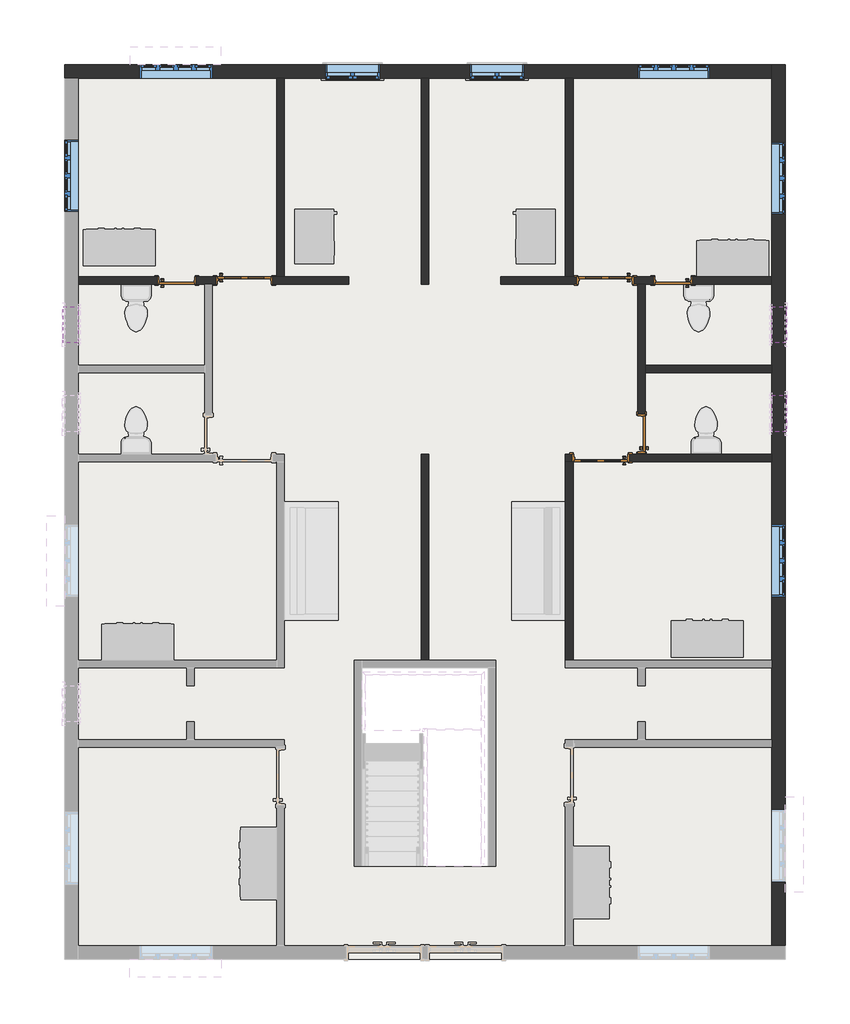
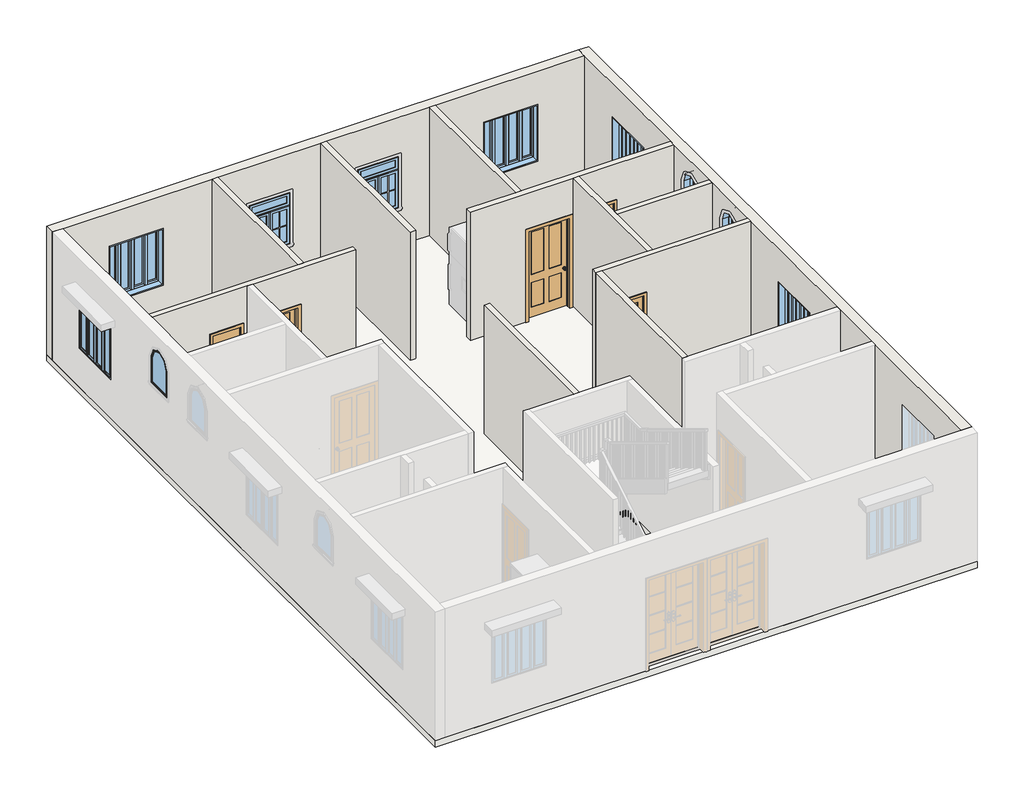
# One storey, part 2 of 4: 12 walls, 10 windows, 6 doors, 1 slab.
"""IFC4 building model written with IfcOpenShell, lengths in millimetres."""

from ifc_helpers import new_model, si_unit, frame, origin, origin_with_axes, place, context, project, spatial, polyline, circle_curve, outline, extrude, faceted_brep, transform, mapped, element, save
from ifc_brep_helpers import plane_surface, revolved_surface, advanced_brep
from components import door_a823658d, door_68a706ac, door_3f5f64ee, door_428b1ac9, window_casement_double_transom_0fae6a54, window_casement_multi_sash_horizontal_main_windows_4_x_7_0e27d311, window_2fd4accf

model = new_model("IFC4")

# Units and contexts
model_context = context("Model", 3, world=origin())
ifc_project = project(units=[si_unit("LENGTHUNIT", "METRE", prefix="MILLI")], contexts=[model_context])

# Site, building, storey
site = spatial("IfcSite", under=ifc_project)
building = spatial("IfcBuilding", under=site)
storey = spatial("IfcBuildingStorey", under=building, Elevation=0.0)

# Doors
placement = place(None, origin())
door_shape = door_a823658d(model_context)
element("IfcDoor", 1, ObjectType="Door-Interior-Single-4_Panel-Wood : 36\" x 84\"", at=placement, inside=storey, context=model_context, shape_type="MappedRepresentation", body=[
    mapped(door_shape, transform((-6490.9771954, 4939.0022103, 0.0), x_axis=(-1.0, 0.0, 0.0), y_axis=(0.0, -1.0, 0.0), z_axis=(0.0, 0.0, 1.0))),
])
door_2_shape = door_68a706ac(model_context)
element("IfcDoor", 2, ObjectType="Door-Interior-Single-4_Panel-Wood : 36\" x 84\"", at=placement, inside=storey, context=model_context, shape_type="MappedRepresentation", body=[
    mapped(door_2_shape, transform((-6567.1771954, 1935.9816069, 0.0), x_axis=(-1.0, 0.0, 0.0), y_axis=(0.0, -1.0, 0.0), z_axis=(0.0, 0.0, 1.0))),
])
element("IfcDoor", 3, ObjectType="Door-Interior-Single-4_Panel-Wood : 36\" x 84\"", at=placement, inside=storey, context=model_context, shape_type="MappedRepresentation", body=[
    mapped(door_2_shape, transform((-12586.9771954, 4939.0022103, 0.0), x_axis=(1.0, 0.0, 0.0), y_axis=(0.0, 1.0, 0.0), z_axis=(0.0, 0.0, 1.0))),
])
door_3_shape = door_3f5f64ee(model_context)
element("IfcDoor", 4, ObjectType="Door-Interior-Single-Flush_Panel-Wood : 24\" x 84\"", at=placement, inside=storey, context=model_context, shape_type="MappedRepresentation", body=[
    mapped(door_3_shape, transform((-5347.9771954, 4932.6522103, 0.0), x_axis=(-1.0, 0.0, 0.0), y_axis=(0.0, -1.0, 0.0), z_axis=(0.0, 0.0, 1.0))),
])
door_4_shape = door_428b1ac9(model_context)
element("IfcDoor", 5, ObjectType="Door-Interior-Single-Flush_Panel-Wood : 24\" x 84\"", at=placement, inside=storey, context=model_context, shape_type="MappedRepresentation", body=[
    mapped(door_4_shape, transform((-13729.9771954, 4932.6522103, 0.0), x_axis=(1.0, 0.0, 0.0), y_axis=(0.0, 1.0, 0.0), z_axis=(0.0, 0.0, 1.0))),
])
element("IfcDoor", 6, ObjectType="Door-Interior-Single-Flush_Panel-Wood : 24\" x 84\"", at=placement, inside=storey, context=model_context, shape_type="MappedRepresentation", body=[
    mapped(door_4_shape, transform((-5878.2021954, 2345.5566069, 0.0), x_axis=(0.0, 1.0, 0.0), y_axis=(-1.0, 0.0, 0.0), z_axis=(0.0, 0.0, 1.0))),
])

# Slab
element("IfcSlab", 7, ObjectType="MARBLE FLOORING 6\"", at=placement, inside=storey, context=model_context, shape_type="SweptSolid", body=[
    extrude(outline(polyline([(-3455.6771954, 8580.7272103), (-3455.6771954, -6532.2727897), (-15623.8646954, -6532.2727897), (-15623.8646954, 8580.7272103), (-3455.6771954, 8580.7272103)]), holes=[polyline([(-10605.7771954, -4957.4727897), (-8472.1771954, -4957.4727897), (-8472.1771954, -1604.6727897), (-10605.7771954, -1604.6727897), (-10605.7771954, -4957.4727897)])]), frame((0.0, 0.0, -152.4), z_axis=(0.0, 0.0, 1.0), x_axis=(1.0, 0.0, 0.0)), (0.0, 0.0, 1.0), 152.4),
])

# Walls
element("IfcWall", 8, ObjectType="INNER WALL 5\"", at=placement, inside=storey, context=model_context, shape_type="Brep", body=[
    faceted_brep([(-10821.6771954, 4872.3272103, 0.0), (-10821.6771954, 4872.3272103, 3048.0), (-13133.0771954, 4872.3272103, 3048.0), (-13260.0771954, 4872.3272103, 3048.0), (-15395.2646954, 4872.3272103, 3048.0), (-15395.2646954, 4872.3272103, 0.0), (-14060.1771954, 4872.3272103, 0.0), (-14060.1771954, 4872.3272103, 2159.0), (-13399.7771954, 4872.3272103, 2159.0), (-13399.7771954, 4872.3272103, 0.0), (-13260.0771954, 4872.3272103, 0.0), (-13133.0771954, 4872.3272103, 0.0), (-13069.5771954, 4872.3272103, 0.0), (-13069.5771954, 4872.3272103, 2159.0), (-12104.3771954, 4872.3272103, 2159.0), (-12104.3771954, 4872.3272103, 0.0), (-10821.6771954, 4999.3272103, 3048.0), (-10821.6771954, 4999.3272103, 0.0), (-11913.8771954, 4999.3272103, 0.0), (-12040.8771954, 4999.3272103, 0.0), (-12104.3771954, 4999.3272103, 0.0), (-12104.3771954, 4999.3272103, 2159.0), (-13069.5771954, 4999.3272103, 2159.0), (-13069.5771954, 4999.3272103, 0.0), (-13399.7771954, 4999.3272103, 0.0), (-13399.7771954, 4999.3272103, 2159.0), (-14060.1771954, 4999.3272103, 2159.0), (-14060.1771954, 4999.3272103, 0.0), (-15395.2646954, 4999.3272103, 0.0), (-15395.2646954, 4999.3272103, 3048.0), (-12040.8771954, 4999.3272103, 3048.0), (-11913.8771954, 4999.3272103, 3048.0)], [[[0, 1, 2, 3, 4, 5, 6, 7, 8, 9, 10, 11, 12, 13, 14, 15]], [[16, 17, 18, 19, 20, 21, 22, 23, 24, 25, 26, 27, 28, 29, 30, 31]], [[17, 0, 15, 20, 19, 18]], [[5, 28, 27, 6]], [[23, 12, 11, 10, 9, 24]], [[1, 0, 17, 16]], [[5, 4, 29, 28]], [[14, 21, 20, 15]], [[21, 14, 13, 22]], [[22, 13, 12, 23]], [[8, 25, 24, 9]], [[25, 8, 7, 26]], [[26, 7, 6, 27]], [[4, 3, 2, 1, 16, 31, 30, 29]]]),
])
element("IfcWall", 9, ObjectType="INNER WALL 5\"", at=placement, inside=storey, context=model_context, shape_type="Brep", body=[
    faceted_brep([(-8256.2771954, 4872.3272103, 3048.0), (-8256.2771954, 4872.3272103, 0.0), (-6973.5771954, 4872.3272103, 0.0), (-6973.5771954, 4872.3272103, 2159.0), (-6008.3771954, 4872.3272103, 2159.0), (-6008.3771954, 4872.3272103, 0.0), (-5944.8771954, 4872.3272103, 0.0), (-5817.8771954, 4872.3272103, 0.0), (-5678.1771954, 4872.3272103, 0.0), (-5678.1771954, 4872.3272103, 2159.0), (-5017.7771954, 4872.3272103, 2159.0), (-5017.7771954, 4872.3272103, 0.0), (-3684.2771954, 4872.3272103, 0.0), (-3684.2771954, 4872.3272103, 3048.0), (-5817.8771954, 4872.3272103, 3048.0), (-5944.8771954, 4872.3272103, 3048.0), (-8256.2771954, 4999.3272103, 0.0), (-8256.2771954, 4999.3272103, 3048.0), (-7164.0771954, 4999.3272103, 3048.0), (-7037.0771954, 4999.3272103, 3048.0), (-3684.2771954, 4999.3272103, 3048.0), (-3684.2771954, 4999.3272103, 0.0), (-5017.7771954, 4999.3272103, 0.0), (-5017.7771954, 4999.3272103, 2159.0), (-5678.1771954, 4999.3272103, 2159.0), (-5678.1771954, 4999.3272103, 0.0), (-6008.3771954, 4999.3272103, 0.0), (-6008.3771954, 4999.3272103, 2159.0), (-6973.5771954, 4999.3272103, 2159.0), (-6973.5771954, 4999.3272103, 0.0), (-7037.0771954, 4999.3272103, 0.0), (-7164.0771954, 4999.3272103, 0.0)], [[[0, 1, 2, 3, 4, 5, 6, 7, 8, 9, 10, 11, 12, 13, 14, 15]], [[16, 17, 18, 19, 20, 21, 22, 23, 24, 25, 26, 27, 28, 29, 30, 31]], [[1, 16, 31, 30, 29, 2]], [[21, 12, 11, 22]], [[5, 26, 25, 8, 7, 6]], [[1, 0, 17, 16]], [[13, 12, 21, 20]], [[28, 3, 2, 29]], [[3, 28, 27, 4]], [[4, 27, 26, 5]], [[24, 9, 8, 25]], [[9, 24, 23, 10]], [[10, 23, 22, 11]], [[0, 15, 14, 13, 20, 19, 18, 17]]]),
])
element("IfcWall", 10, ObjectType="INNER WALL 5\"", at=placement, inside=storey, context=model_context, shape_type="SweptSolid", body=[
    extrude(outline(polyline([(-12040.8771954, 4999.3272103), (-12040.8771954, 8352.1272103), (-11913.8771954, 8352.1272103), (-11913.8771954, 4999.3272103), (-12040.8771954, 4999.3272103)])), origin_with_axes(), (0.0, 0.0, 1.0), 3048.0),
])
element("IfcWall", 11, ObjectType="INNER WALL 5\"", at=placement, inside=storey, context=model_context, shape_type="SweptSolid", body=[
    extrude(outline(polyline([(-9602.4771954, 4872.3272103), (-9602.4771954, 8352.1272103), (-9475.4771954, 8352.1272103), (-9475.4771954, 4872.3272103), (-9602.4771954, 4872.3272103)])), origin_with_axes(), (0.0, 0.0, 1.0), 3048.0),
])
element("IfcWall", 12, ObjectType="INNER WALL 5\"", at=placement, inside=storey, context=model_context, shape_type="SweptSolid", body=[
    extrude(outline(polyline([(-7164.0771954, 4999.3272103), (-7164.0771954, 8352.1272103), (-7037.0771954, 8352.1272103), (-7037.0771954, 4999.3272103), (-7164.0771954, 4999.3272103)])), origin_with_axes(), (0.0, 0.0, 1.0), 3048.0),
])
element("IfcWall", 13, ObjectType="INNER WALL 5\"", at=placement, inside=storey, context=model_context, shape_type="SweptSolid", body=[
    extrude(outline(polyline([(-9602.4771954, -1477.6727897), (-9602.4771954, 2002.6566069), (-9475.4771954, 2002.6566069), (-9475.4771954, -1477.6727897), (-9602.4771954, -1477.6727897)])), origin_with_axes(), (0.0, 0.0, 1.0), 3048.0),
])
element("IfcWall", 14, ObjectType="INNER WALL 5\"", at=placement, inside=storey, context=model_context, shape_type="Brep", body=[
    faceted_brep([(-5944.8771954, 4872.3272103, 3048.0), (-5944.8771954, 4872.3272103, 0.0), (-5944.8771954, 2675.7566069, 0.0), (-5944.8771954, 2675.7566069, 2159.0), (-5944.8771954, 2015.3566069, 2159.0), (-5944.8771954, 2015.3566069, 0.0), (-5944.8771954, 2002.6566069, 0.0), (-5944.8771954, 2002.6566069, 3048.0), (-5817.8771954, 4872.3272103, 0.0), (-5817.8771954, 4872.3272103, 3048.0), (-5817.8771954, 3500.7272103, 3048.0), (-5817.8771954, 3373.7272103, 3048.0), (-5817.8771954, 2002.6566069, 3048.0), (-5817.8771954, 2002.6566069, 0.0), (-5817.8771954, 2015.3566069, 0.0), (-5817.8771954, 2015.3566069, 2159.0), (-5817.8771954, 2675.7566069, 2159.0), (-5817.8771954, 2675.7566069, 0.0), (-5817.8771954, 3373.7272103, 0.0), (-5817.8771954, 3500.7272103, 0.0)], [[[0, 1, 2, 3, 4, 5, 6, 7]], [[8, 9, 10, 11, 12, 13, 14, 15, 16, 17, 18, 19]], [[1, 8, 19, 18, 17, 2]], [[13, 6, 5, 14]], [[1, 0, 9, 8]], [[7, 6, 13, 12]], [[16, 3, 2, 17]], [[3, 16, 15, 4]], [[4, 15, 14, 5]], [[0, 7, 12, 11, 10, 9]]]),
])
element("IfcWall", 15, ObjectType="INNER WALL 5\"", at=placement, inside=storey, context=model_context, shape_type="SweptSolid", body=[
    extrude(outline(polyline([(-3684.2771954, 3373.7272103), (-5817.8771954, 3373.7272103), (-5817.8771954, 3500.7272103), (-3684.2771954, 3500.7272103), (-3684.2771954, 3373.7272103)])), origin_with_axes(), (0.0, 0.0, 1.0), 3048.0),
])
element("IfcWall", 16, ObjectType="INNER WALL 5\"", at=placement, inside=storey, context=model_context, shape_type="Brep", body=[
    faceted_brep([(-3684.2771954, 2002.6566069, 3048.0), (-3684.2771954, 2002.6566069, 0.0), (-5817.8771954, 2002.6566069, 0.0), (-5944.8771954, 2002.6566069, 0.0), (-6084.5771954, 2002.6566069, 0.0), (-6084.5771954, 2002.6566069, 2159.0), (-7049.7771954, 2002.6566069, 2159.0), (-7049.7771954, 2002.6566069, 0.0), (-7164.0771954, 2002.6566069, 0.0), (-7164.0771954, 2002.6566069, 3048.0), (-5944.8771954, 2002.6566069, 3048.0), (-5817.8771954, 2002.6566069, 3048.0), (-3684.2771954, 1875.6566069, 0.0), (-3684.2771954, 1875.6566069, 3048.0), (-7037.0771954, 1875.6566069, 3048.0), (-7164.0771954, 1875.6566069, 3048.0), (-7164.0771954, 1875.6566069, 0.0), (-7049.7771954, 1875.6566069, 0.0), (-7049.7771954, 1875.6566069, 2159.0), (-6084.5771954, 1875.6566069, 2159.0), (-6084.5771954, 1875.6566069, 0.0)], [[[0, 1, 2, 3, 4, 5, 6, 7, 8, 9, 10, 11]], [[12, 13, 14, 15, 16, 17, 18, 19, 20]], [[1, 12, 20, 4, 3, 2]], [[16, 8, 7, 17]], [[1, 0, 13, 12]], [[9, 8, 16, 15]], [[6, 18, 17, 7]], [[18, 6, 5, 19]], [[19, 5, 4, 20]], [[0, 11, 10, 9, 15, 14, 13]]]),
])
element("IfcWall", 17, ObjectType="INNER WALL 5\"", at=placement, inside=storey, context=model_context, shape_type="SweptSolid", body=[
    extrude(outline(polyline([(-7037.0771954, 1875.6566069), (-7037.0771954, -1477.6727897), (-7164.0771954, -1477.6727897), (-7164.0771954, 1875.6566069), (-7037.0771954, 1875.6566069)])), origin_with_axes(), (0.0, 0.0, 1.0), 3048.0),
])
element("IfcWall", 18, ObjectType="OUTER WALL 9\"", at=placement, inside=storey, context=model_context, shape_type="Brep", body=[
    faceted_brep([(-15623.8646954, 8352.1272103, 0.0), (-15395.2646954, 8352.1272103, 0.0), (-12040.8771954, 8352.1272103, 0.0), (-11913.8771954, 8352.1272103, 0.0), (-9602.4771954, 8352.1272103, 0.0), (-9475.4771954, 8352.1272103, 0.0), (-7164.0771954, 8352.1272103, 0.0), (-7037.0771954, 8352.1272103, 0.0), (-3684.2771954, 8352.1272103, 0.0), (-3684.2771954, 8352.1272103, 3048.0), (-7037.0771954, 8352.1272103, 3048.0), (-7164.0771954, 8352.1272103, 3048.0), (-9475.4771954, 8352.1272103, 3048.0), (-9602.4771954, 8352.1272103, 3048.0), (-11913.8771954, 8352.1272103, 3048.0), (-12040.8771954, 8352.1272103, 3048.0), (-15395.2646954, 8352.1272103, 3048.0), (-15623.8646954, 8352.1272103, 3048.0), (-13133.8709454, 8352.1272103, 2260.6), (-13133.8709454, 8352.1272103, 914.4), (-14353.0709454, 8352.1272103, 914.4), (-14353.0709454, 8352.1272103, 2260.6), (-4725.6771954, 8352.1272103, 2260.6), (-4725.6771954, 8352.1272103, 914.4), (-5944.8771954, 8352.1272103, 914.4), (-5944.8771954, 8352.1272103, 2260.6), (-10300.9771954, 8352.1272103, 2133.6), (-10300.9771954, 8352.1272103, 914.4), (-11215.3771954, 8352.1272103, 914.4), (-11215.3771954, 8352.1272103, 2133.6), (-7862.5771954, 8352.1272103, 2133.6), (-7862.5771954, 8352.1272103, 914.4), (-8776.9771954, 8352.1272103, 914.4), (-8776.9771954, 8352.1272103, 2133.6), (-15623.8646954, 8580.7272103, 0.0), (-15623.8646954, 8580.7272103, 3048.0), (-3684.2771954, 8580.7272103, 3048.0), (-3684.2771954, 8580.7272103, 0.0), (-13133.8709454, 8580.7272103, 2260.6), (-14353.0709454, 8580.7272103, 2260.6), (-14353.0709454, 8580.7272103, 914.4), (-13133.8709454, 8580.7272103, 914.4), (-4725.6771954, 8580.7272103, 2260.6), (-5944.8771954, 8580.7272103, 2260.6), (-5944.8771954, 8580.7272103, 914.4), (-4725.6771954, 8580.7272103, 914.4), (-10300.9771954, 8580.7272103, 2133.6), (-11215.3771954, 8580.7272103, 2133.6), (-11215.3771954, 8580.7272103, 914.4), (-10300.9771954, 8580.7272103, 914.4), (-7862.5771954, 8580.7272103, 2133.6), (-8776.9771954, 8580.7272103, 2133.6), (-8776.9771954, 8580.7272103, 914.4), (-7862.5771954, 8580.7272103, 914.4)], [[[0, 1, 2, 3, 4, 5, 6, 7, 8, 9, 10, 11, 12, 13, 14, 15, 16, 17], [18, 19, 20, 21], [22, 23, 24, 25], [26, 27, 28, 29], [30, 31, 32, 33]], [[34, 35, 36, 37], [38, 39, 40, 41], [42, 43, 44, 45], [46, 47, 48, 49], [50, 51, 52, 53]], [[8, 7, 6, 5, 4, 3, 2, 1, 0, 34, 37]], [[0, 17, 35, 34]], [[9, 8, 37, 36]], [[19, 18, 38, 41]], [[20, 19, 41, 40]], [[21, 20, 40, 39]], [[18, 21, 39, 38]], [[23, 22, 42, 45]], [[24, 23, 45, 44]], [[25, 24, 44, 43]], [[22, 25, 43, 42]], [[27, 26, 46, 49]], [[28, 27, 49, 48]], [[29, 28, 48, 47]], [[26, 29, 47, 46]], [[31, 30, 50, 53]], [[32, 31, 53, 52]], [[33, 32, 52, 51]], [[30, 33, 51, 50]], [[17, 16, 15, 14, 13, 12, 11, 10, 9, 36, 35]]]),
])
element("IfcWall", 19, ObjectType="OUTER WALL 9\"", at=placement, inside=storey, context=model_context, shape_type="AdvancedBrep", body=[
    advanced_brep(
    [(-3684.2771954, 8580.7272103, 0.0), (-3684.2771954, 8352.1272103, 0.0), (-3684.2771954, 4999.3272103, 0.0), (-3684.2771954, 4872.3272103, 0.0), (-3684.2771954, 3500.7272103, 0.0), (-3684.2771954, 3373.7272103, 0.0), (-3684.2771954, 2002.6566069, 0.0), (-3684.2771954, 1875.6566069, 0.0), (-3684.2771954, -1477.6727897, 0.0), (-3684.2771954, -1604.6727897, 0.0), (-3684.2771954, -2823.8727897, 0.0), (-3684.2771954, -2950.8727897, 0.0), (-3684.2771954, -6303.6727897, 0.0), (-3684.2771954, -6303.6727897, 3048.0), (-3684.2771954, -2950.8727897, 3048.0), (-3684.2771954, -2823.8727897, 3048.0), (-3684.2771954, -1604.6727897, 3048.0), (-3684.2771954, -1477.6727897, 3048.0), (-3684.2771954, 1875.6566069, 3048.0), (-3684.2771954, 2002.6566069, 3048.0), (-3684.2771954, 3373.7272103, 3048.0), (-3684.2771954, 3500.7272103, 3048.0), (-3684.2771954, 4872.3272103, 3048.0), (-3684.2771954, 4999.3272103, 3048.0), (-3684.2771954, 8352.1272103, 3048.0), (-3684.2771954, 8580.7272103, 3048.0), (-3684.2771954, 6053.4272103, 2260.6), (-3684.2771954, 6053.4272103, 914.4), (-3684.2771954, 7272.6272103, 914.4), (-3684.2771954, 7272.6272103, 2260.6), (-3684.2771954, -410.6080914, 2260.6), (-3684.2771954, -410.6080914, 914.4), (-3684.2771954, 808.5919086, 914.4), (-3684.2771954, 808.5919086, 2260.6), (-3684.2771954, -4004.9727897, 2260.6), (-3684.2771954, -5224.1727897, 2260.6), (-3684.2771954, -5224.1727897, 914.4), (-3684.2771954, -4004.9727897, 914.4), (-3684.2771954, 2992.9919086, 1828.8), (-3684.2771954, 2992.9919086, 2438.4), (-3684.2771954, 2383.3919086, 2438.4), (-3684.2771954, 2383.3919086, 1828.8), (-3684.2771954, 4491.3272103, 1828.8), (-3684.2771954, 4491.3272103, 2438.4), (-3684.2771954, 3881.7272103, 2438.4), (-3684.2771954, 3881.7272103, 1828.8), (-3455.6771954, 8580.7272103, 0.0), (-3455.6771954, 8580.7272103, 3048.0), (-3455.6771954, -6303.6727897, 3048.0), (-3455.6771954, -6303.6727897, 0.0), (-3455.6771954, 6053.4272103, 2260.6), (-3455.6771954, 7272.6272103, 2260.6), (-3455.6771954, 7272.6272103, 914.4), (-3455.6771954, 6053.4272103, 914.4), (-3455.6771954, -410.6080914, 2260.6), (-3455.6771954, 808.5919086, 2260.6), (-3455.6771954, 808.5919086, 914.4), (-3455.6771954, -410.6080914, 914.4), (-3455.6771954, -4004.9727897, 2260.6), (-3455.6771954, -4004.9727897, 914.4), (-3455.6771954, -5224.1727897, 914.4), (-3455.6771954, -5224.1727897, 2260.6), (-3455.6771954, 2992.9919086, 1828.8), (-3455.6771954, 2383.3919086, 1828.8), (-3455.6771954, 2383.3919086, 2438.4), (-3455.6771954, 2992.9919086, 2438.4), (-3455.6771954, 4491.3272103, 1828.8), (-3455.6771954, 3881.7272103, 1828.8), (-3455.6771954, 3881.7272103, 2438.4), (-3455.6771954, 4491.3272103, 2438.4)],
    [
        (0, 1),
        (1, 2),
        (2, 3),
        (3, 4),
        (4, 5),
        (5, 6),
        (6, 7),
        (7, 8),
        (8, 9),
        (9, 10),
        (10, 11),
        (11, 12),
        (12, 13),
        (13, 14),
        (14, 15),
        (15, 16),
        (16, 17),
        (17, 18),
        (18, 19),
        (19, 20),
        (20, 21),
        (21, 22),
        (22, 23),
        (23, 24),
        (24, 25),
        (25, 0),
        (26, 27),
        (27, 28),
        (28, 29),
        (29, 26),
        (30, 31),
        (31, 32),
        (32, 33),
        (33, 30),
        (34, 35),
        (35, 36),
        (36, 37),
        (37, 34),
        (38, 39),
        (39, 40, circle_curve(frame((-3684.2771954, 2688.1919086, 2438.4), z_axis=(1.0, 0.0, 0.0), x_axis=(0.0, -1.0, 0.0)), 304.8)),
        (40, 41),
        (41, 38),
        (42, 43),
        (43, 44, circle_curve(frame((-3684.2771954, 4186.5272103, 2438.4), z_axis=(1.0, 0.0, 0.0), x_axis=(0.0, -1.0, 0.0)), 304.8)),
        (44, 45),
        (45, 42),
        (46, 47),
        (47, 48),
        (48, 49),
        (49, 46),
        (50, 51),
        (51, 52),
        (52, 53),
        (53, 50),
        (54, 55),
        (55, 56),
        (56, 57),
        (57, 54),
        (58, 59),
        (59, 60),
        (60, 61),
        (61, 58),
        (62, 63),
        (63, 64),
        (64, 65, circle_curve(frame((-3455.6771954, 2688.1919086, 2438.4), z_axis=(-1.0, 0.0, 0.0), x_axis=(0.0, -1.0, 0.0)), 304.8)),
        (65, 62),
        (66, 67),
        (67, 68),
        (68, 69, circle_curve(frame((-3455.6771954, 4186.5272103, 2438.4), z_axis=(-1.0, 0.0, 0.0), x_axis=(0.0, -1.0, 0.0)), 304.8)),
        (69, 66),
        (0, 46),
        (49, 12),
        (25, 47),
        (48, 13),
        (26, 50),
        (53, 27),
        (52, 28),
        (51, 29),
        (30, 54),
        (57, 31),
        (56, 32),
        (55, 33),
        (58, 34),
        (37, 59),
        (36, 60),
        (35, 61),
        (62, 38),
        (41, 63),
        (40, 64),
        (39, 65),
        (66, 42),
        (45, 67),
        (44, 68),
        (43, 69),
    ],
    [
        plane_surface(frame((-3684.2771954, 8466.4272103, 0.0), z_axis=(-1.0, 0.0, 0.0), x_axis=(0.0, -1.0, 0.0))),
        plane_surface(frame((-3455.6771954, 8466.4272103, 0.0), z_axis=(1.0, 0.0, 0.0), x_axis=(0.0, 1.0, 0.0))),
        plane_surface(frame((-3684.2771954, 8466.4272103, 0.0), z_axis=(0.0, 0.0, -1.0), x_axis=(1.0, 0.0, 0.0))),
        plane_surface(frame((-15509.5646954, 8580.7272103, 0.0), z_axis=(0.0, 1.0, 0.0), x_axis=(-1.0, 0.0, 0.0))),
        plane_surface(frame((-3569.9771954, -6303.6727897, 0.0), z_axis=(0.0, -1.0, 0.0), x_axis=(-1.0, 0.0, 0.0))),
        plane_surface(frame((-3684.2771954, 6053.4272103, 2260.6), z_axis=(0.0, 1.0, 0.0), x_axis=(1.0, 0.0, 0.0))),
        plane_surface(frame((-3684.2771954, 6053.4272103, 914.4), z_axis=(0.0, 0.0, 1.0), x_axis=(1.0, 0.0, 0.0))),
        plane_surface(frame((-3684.2771954, 7272.6272103, 914.4), z_axis=(0.0, -1.0, 0.0), x_axis=(1.0, 0.0, 0.0))),
        plane_surface(frame((-3684.2771954, 7272.6272103, 2260.6), z_axis=(0.0, 0.0, -1.0), x_axis=(1.0, 0.0, 0.0))),
        plane_surface(frame((-3684.2771954, -410.6080914, 2260.6), z_axis=(0.0, 1.0, 0.0), x_axis=(1.0, 0.0, 0.0))),
        plane_surface(frame((-3684.2771954, -410.6080914, 914.4), z_axis=(0.0, 0.0, 1.0), x_axis=(1.0, 0.0, 0.0))),
        plane_surface(frame((-3684.2771954, 808.5919086, 914.4), z_axis=(0.0, -1.0, 0.0), x_axis=(1.0, 0.0, 0.0))),
        plane_surface(frame((-3684.2771954, 808.5919086, 2260.6), z_axis=(0.0, 0.0, -1.0), x_axis=(1.0, 0.0, 0.0))),
        plane_surface(frame((-3455.6771954, -4004.9727897, 2260.6), z_axis=(0.0, -1.0, 0.0), x_axis=(-1.0, 0.0, 0.0))),
        plane_surface(frame((-3455.6771954, -4004.9727897, 914.4), z_axis=(0.0, 0.0, 1.0), x_axis=(-1.0, 0.0, 0.0))),
        plane_surface(frame((-3455.6771954, -5224.1727897, 914.4), z_axis=(0.0, 1.0, 0.0), x_axis=(-1.0, 0.0, 0.0))),
        plane_surface(frame((-3455.6771954, -5224.1727897, 2260.6), z_axis=(0.0, 0.0, -1.0), x_axis=(-1.0, 0.0, 0.0))),
        plane_surface(frame((-3455.6771954, 2992.9919086, 1828.8), z_axis=(0.0, 0.0, 1.0), x_axis=(-1.0, 0.0, 0.0))),
        plane_surface(frame((-3455.6771954, 2383.3919086, 1828.8), z_axis=(0.0, 1.0, 0.0), x_axis=(-1.0, 0.0, 0.0))),
        revolved_surface(polyline([(-3684.2771954, 2383.3919085999996, 2438.4), (-3455.6771954, 2383.3919085999996, 2438.4)]), (-3684.2771954, 2688.1919086, 2438.4), (-1.0, 0.0, 0.0)),
        plane_surface(frame((-3455.6771954, 2992.9919086, 2438.4), z_axis=(0.0, -1.0, 0.0), x_axis=(-1.0, 0.0, 0.0))),
        plane_surface(frame((-3455.6771954, 4491.3272103, 1828.8), z_axis=(0.0, 0.0, 1.0), x_axis=(-1.0, 0.0, 0.0))),
        plane_surface(frame((-3455.6771954, 3881.7272103, 1828.8), z_axis=(0.0, 1.0, 0.0), x_axis=(-1.0, 0.0, 0.0))),
        revolved_surface(polyline([(-3684.2771954, 3881.7272102999996, 2438.4), (-3455.6771954, 3881.7272102999996, 2438.4)]), (-3684.2771954, 4186.5272103, 2438.4), (-1.0, 0.0, 0.0)),
        plane_surface(frame((-3455.6771954, 4491.3272103, 2438.4), z_axis=(0.0, -1.0, 0.0), x_axis=(-1.0, 0.0, 0.0))),
        plane_surface(frame((-15623.8646954, 8580.7272103, 3048.0), z_axis=(0.0, 0.0, 1.0), x_axis=(1.0, 0.0, 0.0))),
    ],
    [
        (0, [[1, 2, 3, 4, 5, 6, 7, 8, 9, 10, 11, 12, 13, 14, 15, 16, 17, 18, 19, 20, 21, 22, 23, 24, 25, 26], [27, 28, 29, 30], [31, 32, 33, 34], [35, 36, 37, 38], [39, 40, 41, 42], [43, 44, 45, 46]]),
        (1, [[47, 48, 49, 50], [51, 52, 53, 54], [55, 56, 57, 58], [59, 60, 61, 62], [63, 64, 65, 66], [67, 68, 69, 70]]),
        (2, [[-12, -11, -10, -9, -8, -7, -6, -5, -4, -3, -2, -1, 71, -50, 72]]),
        (3, [[-26, 73, -47, -71]]),
        (4, [[-13, -72, -49, 74]]),
        (5, [[-27, 75, -54, 76]]),
        (6, [[-28, -76, -53, 77]]),
        (7, [[-29, -77, -52, 78]]),
        (8, [[-30, -78, -51, -75]]),
        (9, [[-31, 79, -58, 80]]),
        (10, [[-32, -80, -57, 81]]),
        (11, [[-33, -81, -56, 82]]),
        (12, [[-34, -82, -55, -79]]),
        (13, [[-59, 83, -38, 84]]),
        (14, [[-60, -84, -37, 85]]),
        (15, [[-61, -85, -36, 86]]),
        (16, [[-62, -86, -35, -83]]),
        (17, [[-63, 87, -42, 88]]),
        (18, [[-64, -88, -41, 89]]),
        (19, [[-65, -89, -40, 90]]),
        (20, [[-66, -90, -39, -87]]),
        (21, [[-67, 91, -46, 92]]),
        (22, [[-68, -92, -45, 93]]),
        (23, [[-69, -93, -44, 94]]),
        (24, [[-70, -94, -43, -91]]),
        (25, [[-25, -24, -23, -22, -21, -20, -19, -18, -17, -16, -15, -14, -74, -48, -73]]),
    ],
),
])

# Windows
window_casement_double_transom_shape = window_casement_double_transom_0fae6a54(model_context)
element("IfcWindow", 20, ObjectType="Window-Casement-Double-Transom", at=placement, inside=storey, context=model_context, shape_type="MappedRepresentation", body=[
    mapped(window_casement_double_transom_shape, transform((-10758.1771954, 8466.4272103, 0.0), x_axis=(1.0, 0.0, 0.0), y_axis=(0.0, 1.0, 0.0), z_axis=(0.0, 0.0, 1.0))),
])
element("IfcWindow", 21, ObjectType="Window-Casement-Double-Transom", at=placement, inside=storey, context=model_context, shape_type="MappedRepresentation", body=[
    mapped(window_casement_double_transom_shape, transform((-8319.7771954, 8466.4272103, 0.0), x_axis=(1.0, 0.0, 0.0), y_axis=(0.0, 1.0, 0.0), z_axis=(0.0, 0.0, 1.0))),
])
window_casement_multi_sash_horizontal_main_windows_4_x_7_shape = window_casement_multi_sash_horizontal_main_windows_4_x_7_0e27d311(model_context)
element("IfcWindow", 22, ObjectType="Window-Casement-Multi-Sash-Horizontal : MAIN WINDOWS 4' X 7'", at=placement, inside=storey, context=model_context, shape_type="MappedRepresentation", body=[
    mapped(window_casement_multi_sash_horizontal_main_windows_4_x_7_shape, transform((-15509.5646954, 6701.1272103, 0.0), x_axis=(0.0, 1.0, 0.0), y_axis=(-1.0, 0.0, 0.0), z_axis=(0.0, 0.0, 1.0))),
])
element("IfcWindow", 23, ObjectType="Window-Casement-Multi-Sash-Horizontal : MAIN WINDOWS 4' X 7'", at=placement, inside=storey, context=model_context, shape_type="MappedRepresentation", body=[
    mapped(window_casement_multi_sash_horizontal_main_windows_4_x_7_shape, transform((-13743.4709454, 8466.4272103, 0.0), x_axis=(1.0, 0.0, 0.0), y_axis=(0.0, 1.0, 0.0), z_axis=(0.0, 0.0, 1.0))),
])
element("IfcWindow", 24, ObjectType="Window-Casement-Multi-Sash-Horizontal : MAIN WINDOWS 4' X 7'", at=placement, inside=storey, context=model_context, shape_type="MappedRepresentation", body=[
    mapped(window_casement_multi_sash_horizontal_main_windows_4_x_7_shape, transform((-5335.2771954, 8466.4272103, 0.0), x_axis=(1.0, 0.0, 0.0), y_axis=(0.0, 1.0, 0.0), z_axis=(0.0, 0.0, 1.0))),
])
element("IfcWindow", 25, ObjectType="Window-Casement-Multi-Sash-Horizontal : MAIN WINDOWS 4' X 7'", at=placement, inside=storey, context=model_context, shape_type="MappedRepresentation", body=[
    mapped(window_casement_multi_sash_horizontal_main_windows_4_x_7_shape, transform((-3569.9771954, 6663.0272103, 0.0), x_axis=(0.0, -1.0, 0.0), y_axis=(1.0, 0.0, 0.0), z_axis=(0.0, 0.0, 1.0))),
])
element("IfcWindow", 26, ObjectType="Window-Casement-Multi-Sash-Horizontal : MAIN WINDOWS 4' X 7'", at=placement, inside=storey, context=model_context, shape_type="MappedRepresentation", body=[
    mapped(window_casement_multi_sash_horizontal_main_windows_4_x_7_shape, transform((-3569.9771954, 198.9919086, 0.0), x_axis=(0.0, -1.0, 0.0), y_axis=(1.0, 0.0, 0.0), z_axis=(0.0, 0.0, 1.0))),
])
window_shape = window_2fd4accf(model_context)
element("IfcWindow", 27, ObjectType="Window-Fixed-Round-Top : 24\" x 36\"", at=placement, inside=storey, context=model_context, shape_type="MappedRepresentation", body=[
    mapped(window_shape, transform((-3569.9771954, 2688.1919086, 914.4), x_axis=(0.0, -1.0, 0.0), y_axis=(1.0, 0.0, 0.0), z_axis=(0.0, 0.0, 1.0))),
])
element("IfcWindow", 28, ObjectType="Window-Fixed-Round-Top : 24\" x 36\"", at=placement, inside=storey, context=model_context, shape_type="MappedRepresentation", body=[
    mapped(window_shape, transform((-3569.9771954, 4186.5272103, 914.4), x_axis=(0.0, -1.0, 0.0), y_axis=(1.0, 0.0, 0.0), z_axis=(0.0, 0.0, 1.0))),
])
element("IfcWindow", 29, ObjectType="Window-Fixed-Round-Top : 24\" x 36\"", at=placement, inside=storey, context=model_context, shape_type="MappedRepresentation", body=[
    mapped(window_shape, transform((-15509.5646954, 4186.5272103, 914.4), x_axis=(0.0, 1.0, 0.0), y_axis=(-1.0, 0.0, 0.0), z_axis=(0.0, 0.0, 1.0))),
])

save(model, "model.ifc")

# Revit data of these elements
# Type "Door-Interior-Single-4_Panel-Wood : 36\" x 84\""
#   Type Mark = "10"
#   Assembly Code = "C1020300"
#   Analytic Construction = "Wooden"
#   Top Rail = 0' - 4 11/16"
#   Thickness = 0' - 1 3/8"
#   Thermal Resistance (R) = 2.5876 (h·ft²·°F)/BTU
#   Swing Angle [instance default] = 90.00°
#   Stiles = 0' - 4 3/4"
#   Rough Width = 3' - 2"
#   Rough Height = 7' - 1"
#   Mullion = 0' - 4 1/2"
#   Lock Rail = 0' - 7 1/2"
#   Height = 7' - 0"
#   Width = 3' - 0"
#   Heat Transfer Coefficient (U) = 0.3865 BTU/(h·ft²·°F)
#   Bottom Rail = 0' - 9 1/8"
#   Trim Material = Cherry
#   Panel Material = Cherry
#   Frame Material = Cherry
#   Door Handle Material = Aluminum
#   Visual Light Transmittance = 0
#   Solar Heat Gain Coefficient = 0
#   Wall Closure = (empty or 0)
#   Function = (empty or 0)
# Type "Door-Interior-Single-Flush_Panel-Wood : 24\" x 84\""
#   Type Mark = "11"
#   Assembly Code = "C1020300"
#   Analytic Construction = "Wooden"
#   Thickness = 0' - 1 3/8"
#   Thermal Resistance (R) = 2.5876 (h·ft²·°F)/BTU
#   Swing Angle [instance default] = 90.00°
#   Rough Width = 2' - 2"
#   Rough Height = 7' - 1"
#   Height = 7' - 0"
#   Width = 2' - 0"
#   Heat Transfer Coefficient (U) = 0.3865 BTU/(h·ft²·°F)
#   Trim Material = Cherry
#   Panel Material = Cherry
#   Frame Material = Cherry
#   Door Handle Material = Aluminum
#   Visual Light Transmittance = 0
#   Solar Heat Gain Coefficient = 0
#   Wall Closure = (empty or 0)
#   Function = (empty or 0)
# Type "MARBLE FLOORING 6\""
#   Assembly Code = "B1010"
#   Function = 0
#   Layers, outside or top first: 0' - 6" "Default New Material" (function 1)
# Type "INNER WALL 5\""
#   Assembly Code = "B2010"
#   Layers, outside or top first: 0' - 5" "OUTER WALL PAINT" (function 1)
# Type "OUTER WALL 9\""
#   Assembly Code = "B2010"
#   Layers, outside or top first: 0' - 9" "OUTER WALL PAINT" (function 1)
# Type "Window-Casement-Double-Transom"
#   Type Mark = "23"
#   Fire Rating = "0.5h"
#   Assembly Code = "B2020100"
#   Analytic Construction = "Double glazing - domestic"
#   Window Inset [instance default] = 0' - 0"
#   Wall Thickness [instance default] = 0' - 6"
#   Interior Wall Closure [instance default] = 0' - 2 1/4"
#   Half Width = 1' - 6"
#   Visual Light Transmittance = 0.81
#   Transom Height = 1' - 0"
#   Thermal Resistance (R) = 1.8146 (h·ft²·°F)/BTU
#   Solar Heat Gain Coefficient = 0.76
#   Rough Width = 3' - 0 1/2"
#   Rough Height = 4' - 0 1/2"
#   Open Window Height = 3' - 0"
#   Height = 4' - 0"
#   Heat Transfer Coefficient (U) = 0.5511 BTU/(h·ft²·°F)
#   Frame Extension [instance default] = 0' - 0 1/4"
#   Exterior Wall Closure [instance default] = 0' - 1 1/4"
#   Extension Jamb [instance default] = 0' - 2 1/4"
#   Default Sill Height = 3' - 0"
#   Width = 3' - 0"
#   Muntin Visibility = yes
#   Interior Trim Visibility [instance default] = yes
#   Exterior Trim Visibility [instance default] = yes
#   Extension Jamb Visibility [instance default] = yes
#   Interior Trim Material = Wood - Stained
#   Muntin Pattern = Muntin Pattern_2x2 : Muntin Pattern_2x2
#   Interior Trim = Trim-Window-Interior-Flat : Picture Frame
#   Interior Frame Material = Wood - Stained
#   Glass Panel Material = Glass
#   Exterior Trim Material = Clad - White
#   Exterior Trim = Trim-Window-Exterior-Flat : with Sill
#   Exterior Frame Material = Clad - White
#   Wall Closure = (empty or 0)
# Type "Window-Casement-Multi-Sash-Horizontal : MAIN WINDOWS 4' X 7'"
#   Type Mark = "21"
#   Fire Rating = "0.5h"
#   Assembly Code = "B2020100"
#   Analytic Construction = "Double glazing - domestic"
#   Window Inset [instance default] = 0' - 0 5/8"
#   Wall Thickness [instance default] = 0' - 6"
#   Visual Light Transmittance = 0.81
#   Thermal Resistance (R) = 1.8146 (h·ft²·°F)/BTU
#   Solar Heat Gain Coefficient = 0.76
#   Rough Width = 4' - 0 1/2"
#   Rough Height = 4' - 5 1/2"
#   Open Window Width = 1' - 0"
#   Heat Transfer Coefficient (U) = 0.5511 BTU/(h·ft²·°F)
#   Height = 4' - 5"
#   Frame Gap 3 [instance default] = 0' - 1 83/128"
#   Frame Gap 2 [instance default] = 0' - 0 5/8"
#   Frame Gap 1 = 0' - 1 51/128"
#   Default Sill Height = 3' - 0"
#   Width = 4' - 0"
#   Frame Material = Metal - Aluminum
#   Glass Panel Material = Glass
#   Wall Closure = (empty or 0)
# Type "Window-Fixed-Round-Top : 24\" x 36\""
#   Type Mark = "31"
#   Fire Rating = "0.5h"
#   Assembly Code = "B2020100"
#   Analytic Construction = "Double glazing - domestic"
#   Window Inset [instance default] = 0' - 0"
#   Wall Thickness [instance default] = 0' - 6"
#   Visual Light Transmittance = 0.81
#   Thermal Resistance (R) = 1.8146 (h·ft²·°F)/BTU
#   Solar Heat Gain Coefficient = 0.76
#   Rough Width = 2' - 0 1/2"
#   Rough Height = 3' - 0 1/2"
#   Interior Wall Closure [instance default] = 0' - 2 1/4"
#   Height = 3' - 0"
#   Heat Transfer Coefficient (U) = 0.5511 BTU/(h·ft²·°F)
#   Frame Extension [instance default] = 0' - 0 1/4"
#   Exterior Wall Closure [instance default] = 0' - 1 1/4"
#   Extension Jamb [instance default] = 0' - 2 1/4"
#   Default Sill Height = 3' - 0"
#   Width = 2' - 0"
#   Interior Trim Visibility [instance default] = yes
#   Exterior Trim Visibility [instance default] = yes
#   Extension Jamb Visibility [instance default] = yes
#   Interior Trim Material = Wood - Stained
#   Interior Trim = Trim-Window-Interior-Flat-Arch-Top-Tree_Centered : Picture Frame
#   Interior Frame Material = Wood - Stained
#   Glass Panel Material = Glass
#   Exterior Trim Material = Clad - White
#   Exterior Trim = Trim-Window-Exterior-Flat-Arch-Top-Tree_Centered : with Sill
#   Exterior Frame Material = Clad - White
#   Wall Closure = (empty or 0)
# Elements 1, 2, 3 (IfcDoor, "Door-Interior-Single-4_Panel-Wood : 36\" x 84\"")
#   Swing Angle = 90.00°
#   Phase Created = New Construction
#   Materials on its faces: "Cherry", "Aluminum"
# Elements 4, 5, 6 (IfcDoor, "Door-Interior-Single-Flush_Panel-Wood : 24\" x 84\"")
#   Swing Angle = 90.00°
#   Phase Created = New Construction
#   Materials on its faces: "Cherry", "Aluminum"
# Element 7 (IfcSlab, "MARBLE FLOORING 6\"")
#   Height Offset From Level = 0' - 0"
#   Phase Created = New Construction
#   Materials on its faces: "Default New Material", "outer wall paint 234"
# Elements 8, 9, 10, 11, 12, 13, 14, 15, 16, 17 (IfcWall, "INNER WALL 5\"")
#   Top Offset = 0' - 0"
#   Base Offset = 0' - 0"
#   Unconnected Height = 10' - 0"
#   wall height = 10' - 0"
#   Phase Created = New Construction
#   Base Constraint = 1 GND FLR
#   Materials on its faces: "OUTER WALL PAINT"
# Elements 18, 19 (IfcWall, "OUTER WALL 9\"")
#   Top Offset = 0' - 0"
#   Base Offset = 0' - 0"
#   Unconnected Height = 10' - 0"
#   wall height = 10' - 0"
#   Phase Created = New Construction
#   Base Constraint = 1 GND FLR
#   Materials on its faces: "OUTER WALL PAINT", "outer wall paint 234"
# Element 20 (IfcWindow, "Window-Casement-Double-Transom")
#   Mark = "15"
#   Window Inset = 0' - 0"
#   Interior Wall Closure = 0' - 2 1/4"
#   Frame Extension = 0' - 0 1/4"
#   Exterior Wall Closure = 0' - 1 1/4"
#   Interior Trim Visibility = yes
#   Exterior Trim Visibility = yes
#   Phase Created = New Construction
#   Materials on its faces: "Wood - Stained", "Glass", "Clad - White"
# Element 21 (IfcWindow, "Window-Casement-Double-Transom")
#   Mark = "16"
#   Window Inset = 0' - 0"
#   Interior Wall Closure = 0' - 2 1/4"
#   Frame Extension = 0' - 0 1/4"
#   Exterior Wall Closure = 0' - 1 1/4"
#   Interior Trim Visibility = yes
#   Exterior Trim Visibility = yes
#   Phase Created = New Construction
#   Materials on its faces: "Wood - Stained", "Glass", "Clad - White"
# Element 22 (IfcWindow, "Window-Casement-Multi-Sash-Horizontal : MAIN WINDOWS 4' X 7'")
#   Mark = "7"
#   Window Inset = 0' - 0 5/8"
#   Frame Gap 3 = 0' - 1 83/128"
#   Frame Gap 2 = 0' - 0 5/8"
#   Phase Created = New Construction
#   Materials on its faces: "Metal - Aluminum", "Glass"
# Element 23 (IfcWindow, "Window-Casement-Multi-Sash-Horizontal : MAIN WINDOWS 4' X 7'")
#   Mark = "8"
#   Window Inset = 0' - 0 5/8"
#   Frame Gap 3 = 0' - 1 83/128"
#   Frame Gap 2 = 0' - 0 5/8"
#   Phase Created = New Construction
#   Materials on its faces: "Metal - Aluminum", "Glass"
# Element 24 (IfcWindow, "Window-Casement-Multi-Sash-Horizontal : MAIN WINDOWS 4' X 7'")
#   Mark = "9"
#   Window Inset = 0' - 0 5/8"
#   Frame Gap 3 = 0' - 1 83/128"
#   Frame Gap 2 = 0' - 0 5/8"
#   Phase Created = New Construction
#   Materials on its faces: "Metal - Aluminum", "Glass"
# Element 25 (IfcWindow, "Window-Casement-Multi-Sash-Horizontal : MAIN WINDOWS 4' X 7'")
#   Mark = "10"
#   Window Inset = 0' - 0 5/8"
#   Frame Gap 3 = 0' - 1 83/128"
#   Frame Gap 2 = 0' - 0 5/8"
#   Phase Created = New Construction
#   Materials on its faces: "Metal - Aluminum", "Glass"
# Element 26 (IfcWindow, "Window-Casement-Multi-Sash-Horizontal : MAIN WINDOWS 4' X 7'")
#   Mark = "11"
#   Window Inset = 0' - 0 5/8"
#   Frame Gap 3 = 0' - 1 83/128"
#   Frame Gap 2 = 0' - 0 5/8"
#   Phase Created = New Construction
#   Materials on its faces: "Metal - Aluminum", "Glass"
# Element 27 (IfcWindow, "Window-Fixed-Round-Top : 24\" x 36\"")
#   Mark = "26"
#   Window Inset = 0' - 0"
#   Interior Wall Closure = 0' - 2 1/4"
#   Frame Extension = 0' - 0 1/4"
#   Exterior Wall Closure = 0' - 1 1/4"
#   Interior Trim Visibility = yes
#   Exterior Trim Visibility = yes
#   Phase Created = New Construction
#   Materials on its faces: "Wood - Stained", "Clad - White", "Glass"
# Element 28 (IfcWindow, "Window-Fixed-Round-Top : 24\" x 36\"")
#   Mark = "27"
#   Window Inset = 0' - 0"
#   Interior Wall Closure = 0' - 2 1/4"
#   Frame Extension = 0' - 0 1/4"
#   Exterior Wall Closure = 0' - 1 1/4"
#   Interior Trim Visibility = yes
#   Exterior Trim Visibility = yes
#   Phase Created = New Construction
#   Materials on its faces: "Wood - Stained", "Clad - White", "Glass"
# Element 29 (IfcWindow, "Window-Fixed-Round-Top : 24\" x 36\"")
#   Mark = "29"
#   Window Inset = 0' - 0"
#   Interior Wall Closure = 0' - 2 1/4"
#   Frame Extension = 0' - 0 1/4"
#   Exterior Wall Closure = 0' - 1 1/4"
#   Interior Trim Visibility = yes
#   Exterior Trim Visibility = yes
#   Phase Created = New Construction
#   Materials on its faces: "Wood - Stained", "Clad - White", "Glass"
# Materials
#   "Cherry": class "Wood", colour RGB 226 177 128, transparency 0, Description = "Prunus Serotina", Cost = 0
#   "Aluminum": class "Metal", colour RGB 247 247 247, transparency 0, Description = "Aluminum 6061", Cost = 0
#   "Default New Material": class "Generic", colour RGB 120 120 120, transparency 0, Cost = 0
#   "OUTER WALL PAINT": class "Generic", colour RGB 120 120 120, transparency 0, Cost = 0
#   "Wood - Stained": class "Wood", colour RGB 224 178 126, transparency 0, Cost = 0
#   "Glass": class "Glass", colour RGB 0 128 192, transparency 0.75, Description = "Soda Lime Glass", Cost = 0
#   "Clad - White": class "Wood", colour RGB 242 242 238, transparency 0, Cost = 0
#   "Metal - Aluminum": class "Metal", colour RGB 247 247 247, transparency 0
#   "outer wall paint 234": class "Generic", colour RGB 120 120 120, transparency 0, Cost = 0
